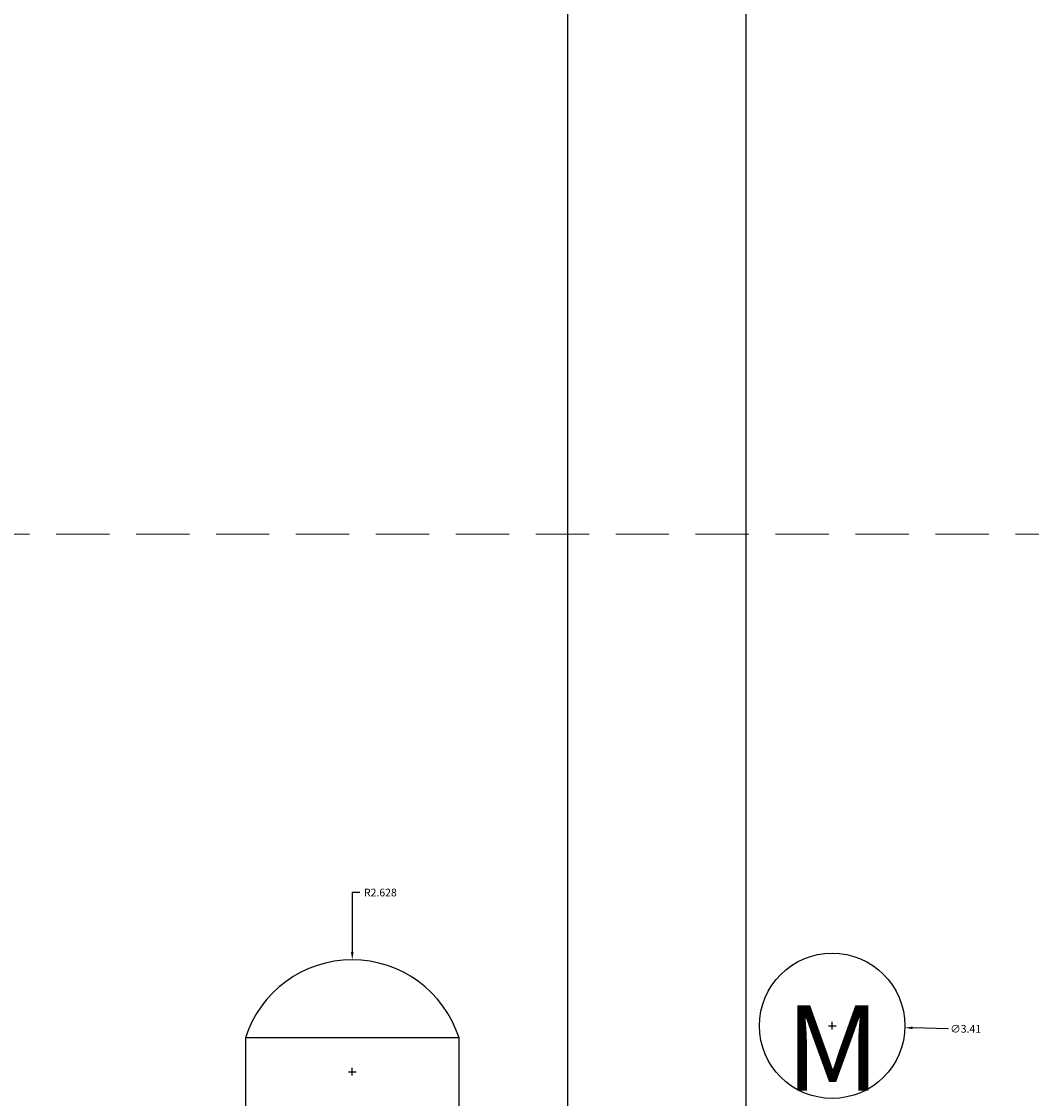
# Model space of a CAD drawing. Units: inches. Extents: x 412 to 584, y 208 to 437.
# Tile 23 of 28: x 471 to 495, y 387 to 412. Entities that reach past the tile are written whole.
import ezdxf

# ---------------------------------------------------------------- set-up
doc = ezdxf.new("R2010")
doc.units = ezdxf.units.IN
doc.header["$MEASUREMENT"] = 0
doc.linetypes.add('HIDDEN', pattern=[0.375, 0.25, -0.125])
for name, color, linetype, lineweight in [('A-ANNO-DIMS', 2, 'Continuous', 18), ('E-ANNO-TEXT', 7, 'Continuous', 18), ('E-ENCL-HIDN', 3, 'HIDDEN', 18), ('E-POWR-EQPM', 3, 'Continuous', 25)]:
    doc.layers.add(name, color=color, linetype=linetype, lineweight=lineweight)
doc.styles.get("Standard").update_dxf_attribs({"font": 'arial.ttf'})
doc.dimstyles.get("Standard").update_dxf_attribs({"dimtxt": 0.18, "dimasz": 0.18, "dimexe": 0.18, "dimexo": 0.0625, "dimgap": 0.09, "dimtad": 0, "dimtih": 1, "dimtoh": 1, "dimdec": 4, "dimzin": 0, "dimdsep": 46, "dimtxsty": 'Standard', "dimcen": 0.09, "dimadec": 0, "dimazin": 0, "dimtfac": 1, "dimtdec": 4, "dimtofl": 0, "dimtmove": 0, "dimatfit": 3, "dimfxl": 1, "dimtolj": 1, "dimtzin": 0, "dimarcsym": 0})

# ---------------------------------------------------------------- blocks, each defined once
blk = doc.blocks.new('*D21')
at = {"layer": 'A-ANNO-DIMS', "color": 0, "lineweight": -2, "transparency": 16777216}
for p, q in [((466.104, 400.237), (466.104, 437.465)), ((538.619, 400.237), (538.619, 437.465)), ((466.284, 437.285), (501.986, 437.285)), ((538.439, 437.285), (502.737, 437.285))]:
    blk.add_line(p, q, dxfattribs=at)
at = {"layer": 'A-ANNO-DIMS', "color": 0, "transparency": 16777216}
for points in [[(466.284, 437.315), (466.284, 437.255), (466.104, 437.285)], [(538.439, 437.315), (538.439, 437.255), (538.619, 437.285)]]:
    blk.add_solid(points, dxfattribs=at)
at = {"layer": 'Defpoints', "color": 0, "transparency": 16777216}
for p in [(538.619, 437.285), (466.104, 400.175), (538.619, 400.175)]:
    blk.add_point(p, dxfattribs=at)
at = {"layer": 'A-ANNO-DIMS', "color": 0, "transparency": 16777216, "insert": (502.361, 437.285), "char_height": 0.18, "attachment_point": 5}
blk.add_mtext('\\A1;72.51', dxfattribs=at)
blk = doc.blocks.new('*D27')
at = {"layer": 'A-ANNO-DIMS', "color": 0, "lineweight": -2, "transparency": 16777216}
for p, q in [((466.104, 400.237), (466.104, 437.465)), ((499.288, 397.825), (499.288, 437.465)), ((466.284, 437.285), (482.233, 437.285)), ((499.108, 437.285), (483.159, 437.285))]:
    blk.add_line(p, q, dxfattribs=at)
at = {"layer": 'A-ANNO-DIMS', "color": 0, "transparency": 16777216}
for points in [[(466.284, 437.315), (466.284, 437.255), (466.104, 437.285)], [(499.108, 437.315), (499.108, 437.255), (499.288, 437.285)]]:
    blk.add_solid(points, dxfattribs=at)
at = {"layer": 'Defpoints', "color": 0, "transparency": 16777216}
for p in [(499.288, 437.285), (466.104, 400.175), (499.288, 397.763)]:
    blk.add_point(p, dxfattribs=at)
at = {"layer": 'A-ANNO-DIMS', "color": 0, "transparency": 16777216, "insert": (482.696, 437.285), "char_height": 0.18, "attachment_point": 5}
blk.add_mtext('\\A1;33.184', dxfattribs=at)
blk = doc.blocks.new('*D28')
at = {"layer": 'A-ANNO-DIMS', "color": 0, "lineweight": -2, "transparency": 16777216}
for p, q in [((450.562, 256.635), (450.562, 437.465)), ((555.796, 256.635), (555.796, 437.465)), ((450.742, 437.285), (502.724, 437.285)), ((555.616, 437.285), (503.634, 437.285))]:
    blk.add_line(p, q, dxfattribs=at)
at = {"layer": 'A-ANNO-DIMS', "color": 0, "transparency": 16777216}
for points in [[(450.742, 437.315), (450.742, 437.255), (450.562, 437.285)], [(555.616, 437.315), (555.616, 437.255), (555.796, 437.285)]]:
    blk.add_solid(points, dxfattribs=at)
at = {"layer": 'Defpoints', "color": 0, "transparency": 16777216}
for p in [(555.796, 437.285), (450.562, 256.573), (555.796, 256.573)]:
    blk.add_point(p, dxfattribs=at)
at = {"layer": 'A-ANNO-DIMS', "color": 0, "transparency": 16777216, "insert": (503.179, 437.285), "char_height": 0.18, "attachment_point": 5}
blk.add_mtext('\\A1;105.23', dxfattribs=at)
blk = doc.blocks.new('*D41')
at = {"layer": 'A-ANNO-DIMS', "color": 0, "lineweight": -2, "transparency": 16777216}
for p, q in [((483.735, 316.045), (483.735, 437.465)), ((487.917, 316.045), (487.917, 437.465)), ((483.915, 437.285), (485.429, 437.285)), ((487.737, 437.285), (486.222, 437.285))]:
    blk.add_line(p, q, dxfattribs=at)
at = {"layer": 'A-ANNO-DIMS', "color": 0, "transparency": 16777216}
for points in [[(483.915, 437.315), (483.915, 437.255), (483.735, 437.285)], [(487.737, 437.315), (487.737, 437.255), (487.917, 437.285)]]:
    blk.add_solid(points, dxfattribs=at)
at = {"layer": 'Defpoints', "color": 0, "transparency": 16777216}
for p in [(487.917, 437.285), (483.735, 315.982), (487.917, 315.982)]:
    blk.add_point(p, dxfattribs=at)
at = {"layer": 'A-ANNO-DIMS', "color": 0, "transparency": 16777216, "insert": (485.826, 437.285), "char_height": 0.18, "attachment_point": 5}
blk.add_mtext('\\A1;4.182', dxfattribs=at)
blk = doc.blocks.new('*D44')
at = {"layer": 'A-ANNO-DIMS', "color": 0, "lineweight": -2, "transparency": 16777216}
for p, q in [((478.854, 391.769), (478.674, 391.769)), ((478.674, 391.769), (478.674, 390.372)), ((478.584, 387.564), (478.764, 387.564)), ((478.674, 387.474), (478.674, 387.654))]:
    blk.add_line(p, q, dxfattribs=at)
at = {"layer": 'A-ANNO-DIMS', "color": 0, "transparency": 16777216}
blk.add_solid([(478.644, 390.372), (478.704, 390.372), (478.674, 390.192)], dxfattribs=at)
at = {"layer": 'Defpoints', "color": 0, "transparency": 16777216}
for p in [(478.674, 390.192), (478.674, 387.564)]:
    blk.add_point(p, dxfattribs=at)
at = {"layer": 'A-ANNO-DIMS', "color": 0, "transparency": 16777216, "insert": (479.334, 391.769), "char_height": 0.18, "attachment_point": 5}
blk.add_mtext('\\A1;R2.628', dxfattribs=at)
blk = doc.blocks.new('*D45')
at = {"layer": 'A-ANNO-DIMS', "color": 0, "lineweight": -2, "transparency": 16777216}
for p, q in [((489.842, 388.644), (490.022, 388.644)), ((489.932, 388.554), (489.932, 388.734)), ((492.659, 388.572), (491.816, 388.594))]:
    blk.add_line(p, q, dxfattribs=at)
at = {"layer": 'A-ANNO-DIMS', "color": 0, "transparency": 16777216}
blk.add_solid([(491.817, 388.624), (491.816, 388.564), (491.637, 388.599)], dxfattribs=at)
at = {"layer": 'Defpoints', "color": 0, "transparency": 16777216}
for p in [(488.228, 388.689), (491.637, 388.599)]:
    blk.add_point(p, dxfattribs=at)
at = {"layer": 'A-ANNO-DIMS', "color": 0, "transparency": 16777216, "insert": (493.064, 388.572), "char_height": 0.18, "attachment_point": 5}
blk.add_mtext('\\A1;∅3.41', dxfattribs=at)

msp = doc.modelspace()

# ---------------------------------------------------------------- linework, layer by layer
at = {"layer": 'E-ENCL-HIDN', "ltscale": 5}
msp.add_lwpolyline([(466.1037, 400.175), (538.6186, 400.175), (538.6186, 360.1961), (466.1037, 360.1961)], close=True, dxfattribs=at)
at = {"layer": 'E-POWR-EQPM'}
msp.add_lwpolyline([(476.1684, 384.6173), (481.1791, 384.6173), (481.1791, 388.3577), (476.1684, 388.3577)], close=True, dxfattribs=at)
msp.add_circle((489.932, 388.6441), 1.7051, dxfattribs=at)
msp.add_arc((478.6738, 387.5639), 2.6281, 17.58033, 162.41967, dxfattribs=at)

# ---------------------------------------------------------------- texts
at = {"layer": 'E-ANNO-TEXT', "insert": (483.1281, 389.1257), "char_height": 2, "attachment_point": 1}
msp.add_mtext_dynamic_manual_height_columns('\\pxqc;M', width=13.633448, gutter_width=1, heights=[2.9648], dxfattribs=at)

# ---------------------------------------------------------------- dimensions: what is measured, and where the dimension line sits
at = {"layer": 'A-ANNO-DIMS'}
for base, p1, p2, override, picture, middle in [((555.7959, 437.2847), (450.562, 256.5729), (555.7959, 256.5729), {"dimdec": 2, "dimlfac": 1, "dimrnd": 0, "dimzin": 0, "dimdsep": 46, "dimlunit": 2}, '*D28', (503.1789, 437.2847)), ((538.6186, 437.2847), (466.1037, 400.175), (538.6186, 400.175), {"dimdec": 2, "dimlfac": 1, "dimrnd": 0, "dimzin": 0, "dimdsep": 46, "dimlunit": 2}, '*D21', (502.3612, 437.2847)), ((499.2878, 437.2847), (466.1037, 400.175), (499.2878, 397.7626), {"dimdec": 3, "dimlfac": 1, "dimrnd": 0, "dimzin": 0, "dimdsep": 46, "dimlunit": 2}, '*D27', (482.6958, 437.2847)), ((487.9167, 437.2847), (483.7347, 315.9821), (487.9167, 315.9821), {"dimdec": 3, "dimlfac": 1, "dimrnd": 0, "dimzin": 0, "dimdsep": 46, "dimlunit": 2}, '*D41', (485.8257, 437.2847))]:
    dim = msp.add_linear_dim(base=base, p1=p1, p2=p2, dimstyle='Standard', override=override, dxfattribs=at)
    dim.commit()
    dim.dimension.update_dxf_attribs({"geometry": picture, "text_midpoint": middle})
dim = msp.add_radius_dim(center=(478.6738, 387.5639), mpoint=(478.674, 390.192), dimstyle='Standard', override={"dimdec": 3, "dimlfac": 1, "dimrnd": 0, "dimzin": 0, "dimdsep": 46, "dimlunit": 2}, dxfattribs=at)
dim.commit()
dim.dimension.update_dxf_attribs({"geometry": '*D44', "text_midpoint": (479.3342, 391.7688), "dimtype": 164})
dim = msp.add_diameter_dim_2p(p1=(488.2275, 388.6892), p2=(491.6365, 388.599), dimstyle='Standard', override={"dimdec": 2, "dimlfac": 1, "dimrnd": 0, "dimzin": 0, "dimdsep": 46, "dimlunit": 2}, dxfattribs=at)
dim.commit()
dim.dimension.update_dxf_attribs({"geometry": '*D45', "text_midpoint": (492.6592, 388.572), "dimtype": 163})

doc.saveas('drawing.dxf')
